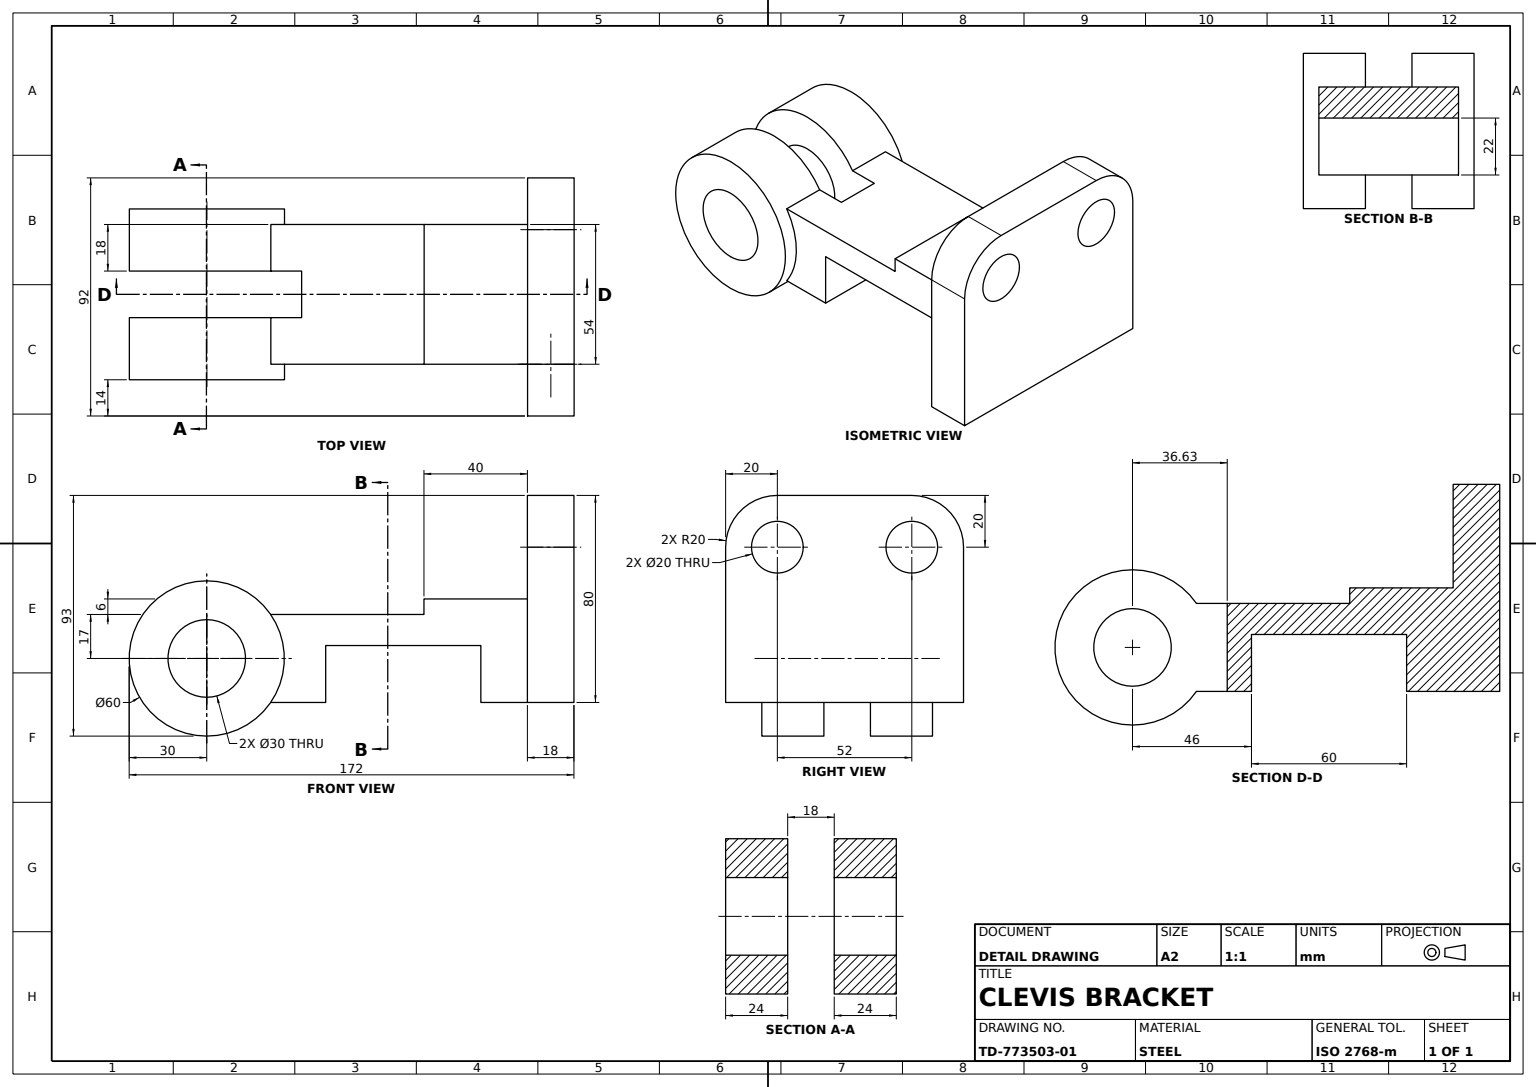
SolidWorks part; units mm, degrees
material "Plain Carbon Steel"
ref_plane "Front Plane" through (0, 0, 0) normal (0, 0, 1) x (1, 0, 0)
ref_plane "Top Plane" through (0, 0, 0) normal (0, 1, 0) x (1, 0, 0)
ref_plane "Right Plane" through (0, 0, 0) normal (1, 0, 0) x (0, 0, -1)
sketch "Mounting Plate Sketch" plane through (0, 0, 0) normal (0, 0, 1) x (1, 0, 0)
  line L1 (0, 0) -> (92, 0)
  line L2 (0, 0) -> (0, 60)
  line L3 (20, 80) -> (72, 80)
  line L4 (92, 0) -> (92, 60)
  circle A0 centre (20, 60) radius 10
  circle A1 centre (72, 60) radius 10
  arc A2 (72, 80) -> (92, 60) centre (72, 60) cw
  arc A3 (0, 60) -> (20, 80) centre (20, 60) cw
  point P11 (92, 80)
  point P14 (0, 80)
  dimension "D7" = 20
  dimension "D8" = 20
  dimension "D1" = 92
  dimension "D2" = 80
  dimension "D3" = 20
  dimension "D4" = 20
  dimension "D5" = 20
  dimension "D6" = 20
extrude "Mounting Plate" add sketch "Mounting Plate Sketch" along normal blind 18
sketch "Arm Sketch 40x40" plane through (92, 0, 0) normal (1, 0, 0) x (0, 0, -1)
  line L1 (-18, 0) -> (-58, 0)
  line L2 (-18, 0) -> (-18, 40)
  line L3 (-18, 40) -> (-58, 40)
  line L4 (-58, 0) -> (-58, 40)
  dimension "D1" = 40
  dimension "D2" = 40
extrude "Arm Boss" add sketch "Arm Sketch 40x40" against normal blind 54 from offset 20 offset against normal yes
sketch "Arm Extension Sketch" plane through (72, 0, 0) normal (1, 0, 0) x (0, 0, -1)
  line L1 (-58, 34) -> (-120, 34)
  line L2 (-120, 34) -> (-120, 0)
  line L3 (-120, 0) -> (-58, 0)
  line L4 (-18, 0) -> (-18, 40)
  line L5 (-18, 40) -> (-58, 40)
  line L6 (-58, 40) -> (-58, 0)
  line L7 (-58, 0) -> (-18, 0)
  line L10 (-58, 34) -> (-58, 0)
  dimension "D2" = 6
  dimension "D3" = 62
  dimension "D1" = 0
extrude "Arm Extension" add sketch "Arm Extension Sketch" against normal blind 54
sketch "Arm Recess Sketch" plane through (72, 0, 0) normal (1, 0, 0) x (0, 0, -1)
  line L0 (-18, 0) -> (-36, 0)
  line L1 (-120, 0) -> (-18, 0) construction
  line L2 (-36, 0) -> (-36, 22)
  line L3 (-36, 22) -> (-96, 22)
  line L4 (-96, 22) -> (-96, 0)
  line L5 (-96, 0) -> (-36, 0)
  line M11 (-120, 0) -> (-18, 0)
  dimension "D1" = 18
  dimension "D2" = 60
  dimension "D3" = 22
extrude "Arm Recess Cut" cut sketch "Arm Recess Sketch" against normal blind 54 contours L3 L4 L2 M11
sketch "Step Pad Sketch" plane through (72, 0, 0) normal (1, 0, 0) x (0, 0, -1)
  line L2 (-118, 52.9593) -> (-118, 7.3901) construction
  line L3 (-142, 17) -> (-96, 17) construction
  line L5 (-96, 22) -> (-96, 0) construction
  line L6 (-96, 17) -> (-57.265, 78.7968) construction
  circle A0 centre (-142, 17) radius 30
  circle A1 centre (-142, 17) radius 15
  dimension "D4" = 60
  dimension "D5" = 30
  dimension "D1" = 46
  dimension "D2" = 17
  dimension "D3" = 24
  dimension "D6" = 45.5692
  dimension "D7" = 9.6099
  dimension "D8" = 72.9332
  dimension "D9" = 122.08
extrude "Step Pad" add sketch "Step Pad Sketch" against normal blind 60 and the other way blind 6
sketch "Clevis Profile Sketch" plane through (0, 0, 0) normal (0, 1, 0) x (1, 0, 0)
  line L0 (45, -172) -> (46, 0) construction
  line L1 (12, -172) -> (78, -172) construction
  line L2 (72, 0) -> (20, 0) construction
  line L3 (18, -117.2816) -> (72, -117.2816) construction
  line L4 (36, -117.2816) -> (54, -117.2816)
  line L5 (36, -117.2816) -> (36, -180.7427)
  line L6 (36, -180.7427) -> (54, -180.7427)
  line L7 (54, -117.2816) -> (54, -180.7427)
  dimension "D1" = 63.4611
  dimension "D2" = 18
  dimension "D3" = 9
extrude "Clevis Profile Cut" cut sketch "Clevis Profile Sketch" against normal through all both and the other way through all contours L5 L4 L7 L6
sketch "Clevis Slot Sketch" plane through (0, 34, 0) normal (0, 1, 0) x (1, 0, 0)
  line L0 (36, -117.2816) -> (36, -105.3725)
  line L2 (54, -117.2816) -> (54, -105.3725)
  line L3 (54, -105.3725) -> (36, -105.3725)
  line L4 (36, -117.2816) -> (54, -117.2816)
  line L6 (18, -117.2816) -> (36, -117.2816) construction
  dimension "D1" = 11.909
extrude "Clevis Slot Cut" cut sketch "Clevis Slot Sketch" against normal through all both
